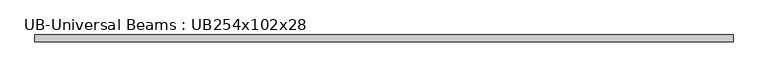
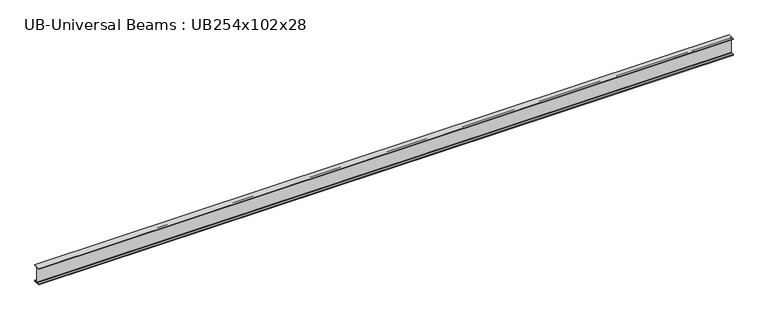
"""IFC4 building model written with IfcOpenShell, lengths in millimetres: beam geometry, UB-Universal Beams : UB254x102x28."""

from ifc_helpers import new_model, si_unit, point, frame, frame_2d, origin, place, context, project, spatial, polyline, circle_curve, trimmed, segment, composite_curve, outline, extrude, source, transform, mapped, element, save


def ub_universal_beams_ub254x102x28_e74905dc(model_context):
    return source(origin(), model_context, "Body", "SweptSolid", [
        extrude(outline(composite_curve([segment(polyline([(51.1, -120.2), (51.1, -130.2), (-51.1, -130.2), (-51.1, -120.2), (-10.75, -120.2)]), True, "CONTINUOUS"), segment(trimmed(circle_curve(frame_2d((-10.75, -112.6)), 7.6), [point((-10.75, -120.2))], [point((-3.15, -112.6))], True, "CARTESIAN"), True, "CONTINUOUS"), segment(polyline([(-3.15, -112.6), (-3.15, 112.6)]), True, "CONTINUOUS"), segment(trimmed(circle_curve(frame_2d((-10.75, 112.6)), 7.6), [point((-3.15, 112.6))], [point((-10.75, 120.2))], True, "CARTESIAN"), True, "CONTINUOUS"), segment(polyline([(-10.75, 120.2), (-51.1, 120.2), (-51.1, 130.2), (51.1, 130.2), (51.1, 120.2), (10.75, 120.2)]), True, "CONTINUOUS"), segment(trimmed(circle_curve(frame_2d((10.75, 112.6)), 7.6), [point((10.75, 120.2))], [point((3.15, 112.6))], True, "CARTESIAN"), True, "CONTINUOUS"), segment(polyline([(3.15, 112.6), (3.15, -112.6)]), True, "CONTINUOUS"), segment(trimmed(circle_curve(frame_2d((10.75, -112.6)), 7.6), [point((3.15, -112.6))], [point((10.75, -120.2))], True, "CARTESIAN"), True, "CONTINUOUS"), segment(polyline([(10.75, -120.2), (51.1, -120.2)]), True, "CONTINUOUS")], self_intersect=False)), frame((-5250.0, 0.0, 0.0), z_axis=(1.0, 0.0, 0.0), x_axis=(0.0, 1.0, 0.0)), (0.0, 0.0, 1.0), 10500.0),
    ])


if __name__ == "__main__":
    model = new_model("IFC4")
    model_context = context("Model", 3, world=origin())
    ifc_project = project(units=[si_unit("LENGTHUNIT", "METRE", prefix="MILLI")], contexts=[model_context])
    site = spatial("IfcSite", under=ifc_project)
    building = spatial("IfcBuilding", under=site)
    placement = place(None, origin())
    ub_universal_beams_ub254x102x28_shape = ub_universal_beams_ub254x102x28_e74905dc(model_context)
    element("IfcBeam", 1, ObjectType="UB-Universal Beams : UB254x102x28", at=placement, inside=building, context=model_context, shape_type="MappedRepresentation", body=[
        mapped(ub_universal_beams_ub254x102x28_shape, transform((0.0, 0.0, 0.0), x_axis=(1.0, 0.0, 0.0), y_axis=(0.0, 1.0, 0.0), z_axis=(0.0, 0.0, 1.0))),
    ])
    save(model, "model.ifc")

# Revit data of these elements
# Type "UB-Universal Beams : UB254x102x28"
#   Section Name Key = "UB254X102X28"
#   Width = 10.22 cm
#   Web Thickness = 0.63 cm
#   Web Fillet = 0.76 cm
#   Warping Constant = 28000.0 cm⁶
#   Torsional Moment of Inertia = 9.57 cm⁴
#   Section Area = 36.1 cm²
#   Plastic Modulus weak axis = 54.8 cm³
#   Plastic Modulus strong axis = 353.0 cm³
#   Nominal Weight = 28.2999 kgf/m
#   Moment of Inertia weak axis = 179.00 cm⁴
#   Moment of Inertia strong axis = 4005.00 cm⁴
#   Height = 26.04 cm
#   Flange Thickness = 1.0 cm
#   Elastic Modulus weak axis = 34.9 cm³
#   Elastic Modulus strong axis = 308.0 cm³
#   Centroid Vertical = 13.02 cm
#   Centroid Horizontal = 5.11 cm
#   Bolt Spacing = 5.4 cm
#   Length [instance default] = 4' - 11.05512"
#   Structural Material [instance default] = Metal - Steel 43-275
#   Type Comments = ""
#   Assembly Code = ""
# Element 1 (IfcBeam, "UB-Universal Beams : UB254x102x28")
#   Materials on its faces: "Metal - Steel 43-275"
# Materials
#   "Metal - Steel 43-275": class "Metal", colour RGB 247 247 247, transparency 0, Cost = 0
